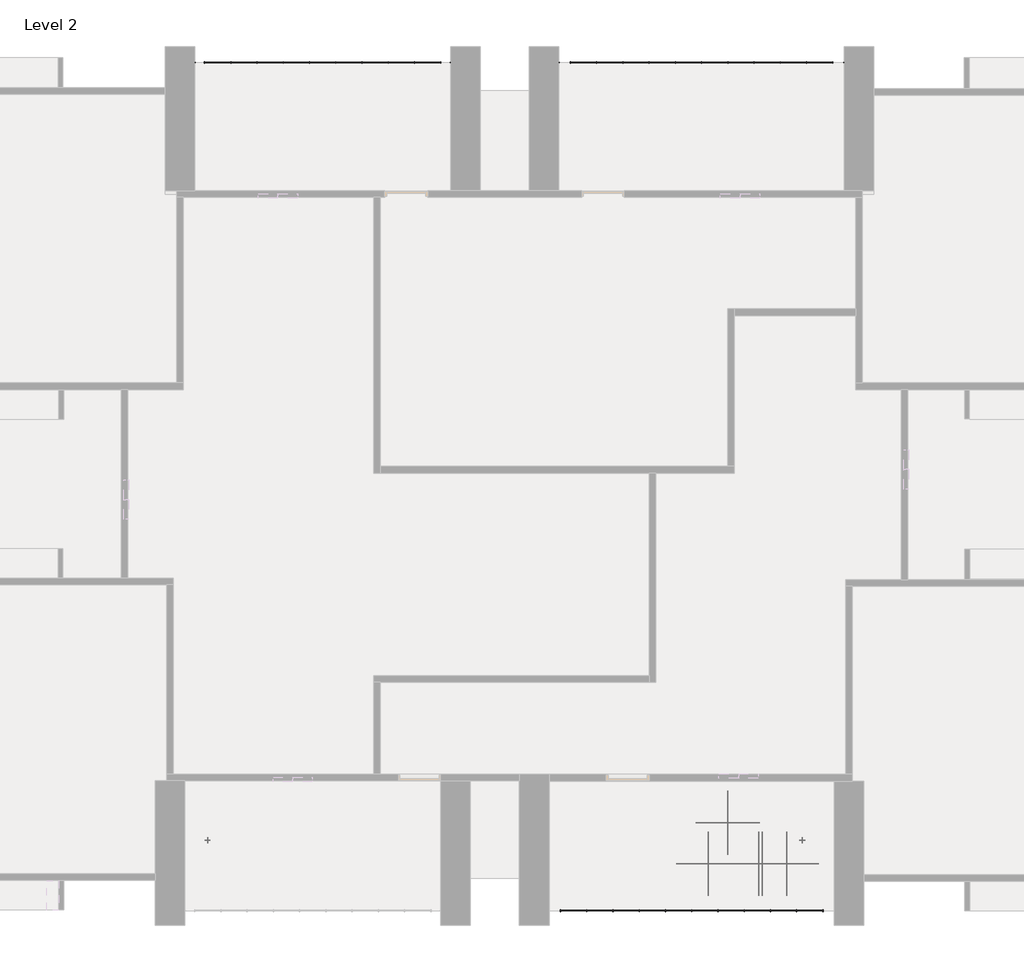
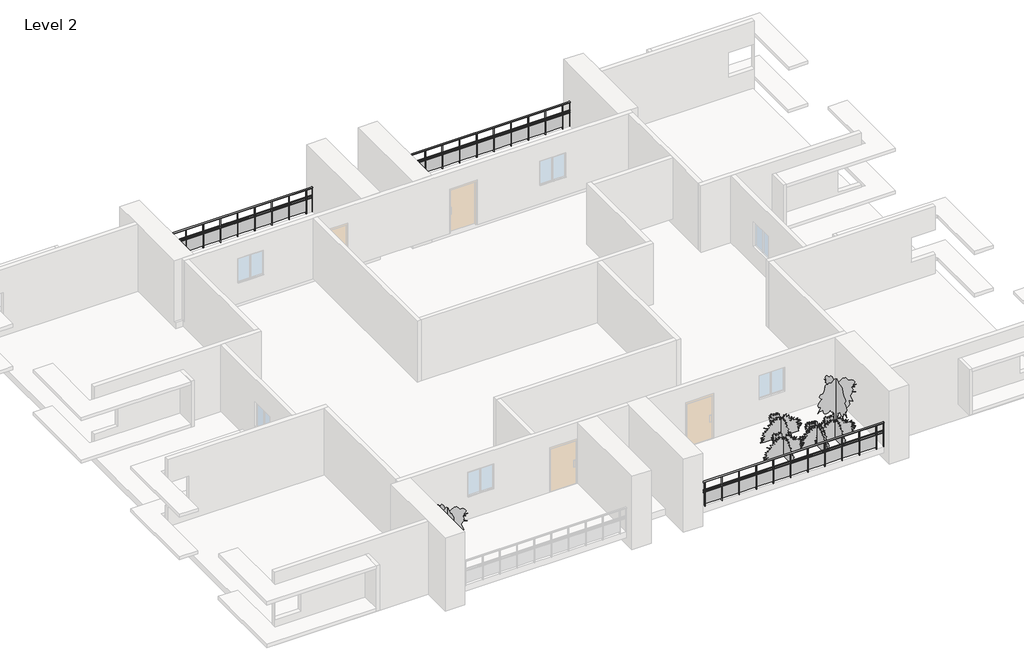
# One storey, part 4 of 4: 7 geographic elements, 3 railings.
"""IFC4 building model written with IfcOpenShell, lengths in millimetres."""

from ifc_helpers import new_model, si_unit, point, frame, origin, place, context, project, spatial, polyline, ellipse_curve, trimmed, outline, extrude, transform, mapped, element, save
from ifc_brep_helpers import plane_surface, extruded_surface, advanced_brep
from components import geographic_element_3d6ded1d, rpc_tree_tropical_d7a905c7

model = new_model("IFC4")

# Units and contexts
model_context = context("Model", 3, world=origin())
ifc_project = project(units=[si_unit("LENGTHUNIT", "METRE", prefix="MILLI")], contexts=[model_context])

# Site, building, storey
site = spatial("IfcSite", under=ifc_project)
building = spatial("IfcBuilding", under=site)
storey = spatial("IfcBuildingStorey", under=building, Name="Level 2", Elevation=3048.0)

# Geographic elements
placement = place(None, origin())
geographic_element_shape = geographic_element_3d6ded1d(model_context)
element("IfcGeographicElement", 1, ObjectType="RPC Shrub : Fountain Grass 3'-6\"", at=placement, inside=storey, context=model_context, shape_type="MappedRepresentation", body=[
    mapped(geographic_element_shape, transform((9500.2520665, -7929.230811, 3657.6), x_axis=(1.0, 0.0, 0.0), y_axis=(0.0, 1.0, 0.0), z_axis=(0.0, 0.0, 1.0))),
])
element("IfcGeographicElement", 2, ObjectType="RPC Shrub : Fountain Grass 3'-6\"", at=placement, inside=storey, context=model_context, shape_type="MappedRepresentation", body=[
    mapped(geographic_element_shape, transform((11938.6520665, -7929.230811, 3657.6), x_axis=(1.0, 0.0, 0.0), y_axis=(0.0, 1.0, 0.0), z_axis=(0.0, 0.0, 1.0))),
])
element("IfcGeographicElement", 3, ObjectType="RPC Shrub : Fountain Grass 3'-6\"", at=placement, inside=storey, context=model_context, shape_type="MappedRepresentation", body=[
    mapped(geographic_element_shape, transform((11176.6520665, -7929.230811, 3657.6), x_axis=(1.0, 0.0, 0.0), y_axis=(0.0, 1.0, 0.0), z_axis=(0.0, 0.0, 1.0))),
])
element("IfcGeographicElement", 4, ObjectType="RPC Shrub : Fountain Grass 3'-6\"", at=placement, inside=storey, context=model_context, shape_type="MappedRepresentation", body=[
    mapped(geographic_element_shape, transform((11075.0520665, -7929.230811, 3657.6), x_axis=(1.0, 0.0, 0.0), y_axis=(0.0, 1.0, 0.0), z_axis=(0.0, 0.0, 1.0))),
])
element("IfcGeographicElement", 5, ObjectType="RPC Shrub : Fountain Grass 3'-6\"", at=placement, inside=storey, context=model_context, shape_type="MappedRepresentation", body=[
    mapped(geographic_element_shape, transform((10109.8520665, -6659.230811, 3657.6), x_axis=(1.0, 0.0, 0.0), y_axis=(0.0, 1.0, 0.0), z_axis=(0.0, 0.0, 1.0))),
])
rpc_tree_tropical_shape = rpc_tree_tropical_d7a905c7(model_context)
element("IfcGeographicElement", 6, ObjectType="RPC Tree - Tropical", at=placement, inside=storey, context=model_context, shape_type="MappedRepresentation", body=[
    mapped(rpc_tree_tropical_shape, transform((-5993.7479335, -7192.630811, 3657.6), x_axis=(1.0, 0.0, 0.0), y_axis=(0.0, 1.0, 0.0), z_axis=(0.0, 0.0, 1.0))),
])
element("IfcGeographicElement", 7, ObjectType="RPC Tree - Tropical", at=placement, inside=storey, context=model_context, shape_type="MappedRepresentation", body=[
    mapped(rpc_tree_tropical_shape, transform((12421.2520665, -7192.630811, 3657.6), x_axis=(1.0, 0.0, 0.0), y_axis=(0.0, 1.0, 0.0), z_axis=(0.0, 0.0, 1.0))),
])

# Railings
element("IfcRailing", 8, ObjectType="Glass Panel - Bottom Fill", at=placement, inside=storey, context=model_context, shape_type="SolidModel", body=[
    advanced_brep(
    [(4572.6520665, -9342.282663, 4876.8), (4572.6520665, -9418.482663, 4876.8), (13411.8520665, -9342.282663, 4876.8), (13411.8520665, -9418.482663, 4876.8)],
    [
        (0, 1, ellipse_curve(frame((4572.6520665, -9380.382663, 4876.8), z_axis=(-1.0, 0.0, 0.0), x_axis=(0.0, -1.0, 0.0)), 38.1, 28.575)),
        (1, 0, ellipse_curve(frame((4572.6520665, -9380.382663, 4876.8), z_axis=(-1.0, 0.0, 0.0), x_axis=(0.0, -1.0, 0.0)), 38.1, 28.575)),
        (2, 3, ellipse_curve(frame((13411.8520665, -9380.382663, 4876.8), z_axis=(1.0, 0.0, 0.0), x_axis=(0.0, -1.0, 0.0)), 38.1, 28.575)),
        (3, 2, ellipse_curve(frame((13411.8520665, -9380.382663, 4876.8), z_axis=(1.0, 0.0, 0.0), x_axis=(0.0, -1.0, 0.0)), 38.1, 28.575)),
        (0, 2),
        (3, 1),
    ],
    [
        plane_surface(frame((4572.6520665, -9380.382663, 4876.8), z_axis=(-1.0, 0.0, 0.0), x_axis=(0.0, 1.0, 0.0))),
        plane_surface(frame((13411.8520665, -9380.382663, 4876.8), z_axis=(1.0, 0.0, 0.0), x_axis=(0.0, 1.0, 0.0))),
        extruded_surface(trimmed(ellipse_curve(frame((13411.8520665, -9380.382663, 4876.8), z_axis=(-1.0, 0.0, 0.0), x_axis=(0.0, -1.0, 0.0)), 38.1, 28.575), [point((13411.8520665, -9342.282663, 4876.8))], [point((13411.8520665, -9418.482663, 4876.8))], True, "CARTESIAN"), (-8839.2, 0.0, 0.0), 8839.2),
        extruded_surface(trimmed(ellipse_curve(frame((13411.8520665, -9380.382663, 4876.8), z_axis=(-1.0, 0.0, 0.0), x_axis=(0.0, -1.0, 0.0)), 38.1, 28.575), [point((13411.8520665, -9418.482663, 4876.8))], [point((13411.8520665, -9342.282663, 4876.8))], True, "CARTESIAN"), (-8839.2, 0.0, 0.0), 8839.2),
    ],
    [
        (0, [[1, 2]]),
        (1, [[3, 4]]),
        (2, [[-1, 5, -4, 6]]),
        (3, [[-2, -6, -3, -5]]),
    ],
),
    extrude(outline(polyline([(4572.6520665, -9393.082663), (4572.6520665, -9367.682663), (13411.8520665, -9367.682663), (13411.8520665, -9393.082663), (4572.6520665, -9393.082663)])), frame((0.0, 0.0, 4457.7), z_axis=(0.0, 0.0, 1.0), x_axis=(1.0, 0.0, 0.0)), (0.0, 0.0, 1.0), 25.4),
    extrude(outline(polyline([(4572.6520665, -9393.082663), (4572.6520665, -9367.682663), (13411.8520665, -9367.682663), (13411.8520665, -9393.082663), (4572.6520665, -9393.082663)])), frame((0.0, 0.0, 4356.1), z_axis=(0.0, 0.0, 1.0), x_axis=(1.0, 0.0, 0.0)), (0.0, 0.0, 1.0), 25.4),
    extrude(outline(polyline([(13049.9020665, -9405.782663), (13049.9020665, -9354.982663), (13062.6020665, -9354.982663), (13062.6020665, -9405.782663), (13049.9020665, -9405.782663)])), frame((0.0, 0.0, 3657.6), z_axis=(0.0, 0.0, 1.0), x_axis=(1.0, 0.0, 0.0)), (0.0, 0.0, 1.0), 1190.4788223),
    extrude(outline(polyline([(12243.4520665, -9373.847506), (13056.2520665, -9373.847506), (13056.2520665, -9380.197506), (12243.4520665, -9380.197506), (12243.4520665, -9373.847506)])), frame((0.0, 0.0, 3759.2), z_axis=(0.0, 0.0, 1.0), x_axis=(1.0, 0.0, 0.0)), (0.0, 0.0, 1.0), 596.9),
    extrude(outline(polyline([(12237.1020665, -9405.782663), (12237.1020665, -9354.982663), (12249.8020665, -9354.982663), (12249.8020665, -9405.782663), (12237.1020665, -9405.782663)])), frame((0.0, 0.0, 3657.6), z_axis=(0.0, 0.0, 1.0), x_axis=(1.0, 0.0, 0.0)), (0.0, 0.0, 1.0), 1190.4788223),
    extrude(outline(polyline([(11430.6520665, -9373.847506), (12243.4520665, -9373.847506), (12243.4520665, -9380.197506), (11430.6520665, -9380.197506), (11430.6520665, -9373.847506)])), frame((0.0, 0.0, 3759.2), z_axis=(0.0, 0.0, 1.0), x_axis=(1.0, 0.0, 0.0)), (0.0, 0.0, 1.0), 596.9),
    extrude(outline(polyline([(11424.3020665, -9405.782663), (11424.3020665, -9354.982663), (11437.0020665, -9354.982663), (11437.0020665, -9405.782663), (11424.3020665, -9405.782663)])), frame((0.0, 0.0, 3657.6), z_axis=(0.0, 0.0, 1.0), x_axis=(1.0, 0.0, 0.0)), (0.0, 0.0, 1.0), 1190.4788223),
    extrude(outline(polyline([(10617.8520665, -9373.847506), (11430.6520665, -9373.847506), (11430.6520665, -9380.197506), (10617.8520665, -9380.197506), (10617.8520665, -9373.847506)])), frame((0.0, 0.0, 3759.2), z_axis=(0.0, 0.0, 1.0), x_axis=(1.0, 0.0, 0.0)), (0.0, 0.0, 1.0), 596.9),
    extrude(outline(polyline([(10611.5020665, -9405.782663), (10611.5020665, -9354.982663), (10624.2020665, -9354.982663), (10624.2020665, -9405.782663), (10611.5020665, -9405.782663)])), frame((0.0, 0.0, 3657.6), z_axis=(0.0, 0.0, 1.0), x_axis=(1.0, 0.0, 0.0)), (0.0, 0.0, 1.0), 1190.4788223),
    extrude(outline(polyline([(9805.0520665, -9373.847506), (10617.8520665, -9373.847506), (10617.8520665, -9380.197506), (9805.0520665, -9380.197506), (9805.0520665, -9373.847506)])), frame((0.0, 0.0, 3759.2), z_axis=(0.0, 0.0, 1.0), x_axis=(1.0, 0.0, 0.0)), (0.0, 0.0, 1.0), 596.9),
    extrude(outline(polyline([(9798.7020665, -9405.782663), (9798.7020665, -9354.982663), (9811.4020665, -9354.982663), (9811.4020665, -9405.782663), (9798.7020665, -9405.782663)])), frame((0.0, 0.0, 3657.6), z_axis=(0.0, 0.0, 1.0), x_axis=(1.0, 0.0, 0.0)), (0.0, 0.0, 1.0), 1190.4788223),
    extrude(outline(polyline([(8992.2520665, -9373.847506), (9805.0520665, -9373.847506), (9805.0520665, -9380.197506), (8992.2520665, -9380.197506), (8992.2520665, -9373.847506)])), frame((0.0, 0.0, 3759.2), z_axis=(0.0, 0.0, 1.0), x_axis=(1.0, 0.0, 0.0)), (0.0, 0.0, 1.0), 596.9),
    extrude(outline(polyline([(8985.9020665, -9405.782663), (8985.9020665, -9354.982663), (8998.6020665, -9354.982663), (8998.6020665, -9405.782663), (8985.9020665, -9405.782663)])), frame((0.0, 0.0, 3657.6), z_axis=(0.0, 0.0, 1.0), x_axis=(1.0, 0.0, 0.0)), (0.0, 0.0, 1.0), 1190.4788223),
    extrude(outline(polyline([(8179.4520665, -9373.847506), (8992.2520665, -9373.847506), (8992.2520665, -9380.197506), (8179.4520665, -9380.197506), (8179.4520665, -9373.847506)])), frame((0.0, 0.0, 3759.2), z_axis=(0.0, 0.0, 1.0), x_axis=(1.0, 0.0, 0.0)), (0.0, 0.0, 1.0), 596.9),
    extrude(outline(polyline([(8173.1020665, -9405.782663), (8173.1020665, -9354.982663), (8185.8020665, -9354.982663), (8185.8020665, -9405.782663), (8173.1020665, -9405.782663)])), frame((0.0, 0.0, 3657.6), z_axis=(0.0, 0.0, 1.0), x_axis=(1.0, 0.0, 0.0)), (0.0, 0.0, 1.0), 1190.4788223),
    extrude(outline(polyline([(7366.6520665, -9373.847506), (8179.4520665, -9373.847506), (8179.4520665, -9380.197506), (7366.6520665, -9380.197506), (7366.6520665, -9373.847506)])), frame((0.0, 0.0, 3759.2), z_axis=(0.0, 0.0, 1.0), x_axis=(1.0, 0.0, 0.0)), (0.0, 0.0, 1.0), 596.9),
    extrude(outline(polyline([(7360.3020665, -9405.782663), (7360.3020665, -9354.982663), (7373.0020665, -9354.982663), (7373.0020665, -9405.782663), (7360.3020665, -9405.782663)])), frame((0.0, 0.0, 3657.6), z_axis=(0.0, 0.0, 1.0), x_axis=(1.0, 0.0, 0.0)), (0.0, 0.0, 1.0), 1190.4788223),
    extrude(outline(polyline([(6553.8520665, -9373.847506), (7366.6520665, -9373.847506), (7366.6520665, -9380.197506), (6553.8520665, -9380.197506), (6553.8520665, -9373.847506)])), frame((0.0, 0.0, 3759.2), z_axis=(0.0, 0.0, 1.0), x_axis=(1.0, 0.0, 0.0)), (0.0, 0.0, 1.0), 596.9),
    extrude(outline(polyline([(6547.5020665, -9405.782663), (6547.5020665, -9354.982663), (6560.2020665, -9354.982663), (6560.2020665, -9405.782663), (6547.5020665, -9405.782663)])), frame((0.0, 0.0, 3657.6), z_axis=(0.0, 0.0, 1.0), x_axis=(1.0, 0.0, 0.0)), (0.0, 0.0, 1.0), 1190.4788223),
    extrude(outline(polyline([(5741.0520665, -9373.847506), (6553.8520665, -9373.847506), (6553.8520665, -9380.197506), (5741.0520665, -9380.197506), (5741.0520665, -9373.847506)])), frame((0.0, 0.0, 3759.2), z_axis=(0.0, 0.0, 1.0), x_axis=(1.0, 0.0, 0.0)), (0.0, 0.0, 1.0), 596.9),
    extrude(outline(polyline([(5734.7020665, -9405.782663), (5734.7020665, -9354.982663), (5747.4020665, -9354.982663), (5747.4020665, -9405.782663), (5734.7020665, -9405.782663)])), frame((0.0, 0.0, 3657.6), z_axis=(0.0, 0.0, 1.0), x_axis=(1.0, 0.0, 0.0)), (0.0, 0.0, 1.0), 1190.4788223),
    extrude(outline(polyline([(4928.2520665, -9373.847506), (5741.0520665, -9373.847506), (5741.0520665, -9380.197506), (4928.2520665, -9380.197506), (4928.2520665, -9373.847506)])), frame((0.0, 0.0, 3759.2), z_axis=(0.0, 0.0, 1.0), x_axis=(1.0, 0.0, 0.0)), (0.0, 0.0, 1.0), 596.9),
    extrude(outline(polyline([(4921.9020665, -9405.782663), (4921.9020665, -9354.982663), (4934.6020665, -9354.982663), (4934.6020665, -9405.782663), (4921.9020665, -9405.782663)])), frame((0.0, 0.0, 3657.6), z_axis=(0.0, 0.0, 1.0), x_axis=(1.0, 0.0, 0.0)), (0.0, 0.0, 1.0), 1190.4788223),
    extrude(outline(polyline([(13399.1520665, -9389.907663), (13399.1520665, -9370.857663), (13418.2020665, -9370.857663), (13418.2020665, -9389.907663), (13399.1520665, -9389.907663)])), frame((0.0, 0.0, 3657.6), z_axis=(0.0, 0.0, 1.0), x_axis=(1.0, 0.0, 0.0)), (0.0, 0.0, 1.0), 1190.4788223),
    extrude(outline(polyline([(4566.3020665, -9389.907663), (4566.3020665, -9370.857663), (4585.3520665, -9370.857663), (4585.3520665, -9389.907663), (4566.3020665, -9389.907663)])), frame((0.0, 0.0, 3657.6), z_axis=(0.0, 0.0, 1.0), x_axis=(1.0, 0.0, 0.0)), (0.0, 0.0, 1.0), 1190.4788223),
])
element("IfcRailing", 9, ObjectType="Glass Panel - Bottom Fill", at=placement, inside=storey, context=model_context, shape_type="SolidModel", body=[
    advanced_brep(
    [(-6400.1479335, 16924.2559451, 4876.8), (-6400.1479335, 16848.0559451, 4876.8), (1524.6520665, 16924.2559451, 4876.8), (1524.6520665, 16848.0559451, 4876.8)],
    [
        (0, 1, ellipse_curve(frame((-6400.1479335, 16886.1559451, 4876.8), z_axis=(-1.0, 0.0, 0.0), x_axis=(0.0, -1.0, 0.0)), 38.1, 28.575)),
        (1, 0, ellipse_curve(frame((-6400.1479335, 16886.1559451, 4876.8), z_axis=(-1.0, 0.0, 0.0), x_axis=(0.0, -1.0, 0.0)), 38.1, 28.575)),
        (2, 3, ellipse_curve(frame((1524.6520665, 16886.1559451, 4876.8), z_axis=(1.0, 0.0, 0.0), x_axis=(0.0, -1.0, 0.0)), 38.1, 28.575)),
        (3, 2, ellipse_curve(frame((1524.6520665, 16886.1559451, 4876.8), z_axis=(1.0, 0.0, 0.0), x_axis=(0.0, -1.0, 0.0)), 38.1, 28.575)),
        (0, 2),
        (3, 1),
    ],
    [
        plane_surface(frame((-6400.1479335, 16886.1559451, 4876.8), z_axis=(-1.0, 0.0, 0.0), x_axis=(0.0, 1.0, 0.0))),
        plane_surface(frame((1524.6520665, 16886.1559451, 4876.8), z_axis=(1.0, 0.0, 0.0), x_axis=(0.0, 1.0, 0.0))),
        extruded_surface(trimmed(ellipse_curve(frame((1524.6520665, 16886.1559451, 4876.8), z_axis=(-1.0, 0.0, 0.0), x_axis=(0.0, -1.0, 0.0)), 38.1, 28.575), [point((1524.6520665, 16924.2559451, 4876.8))], [point((1524.6520665, 16848.0559451, 4876.8))], True, "CARTESIAN"), (-7924.8, 0.0, 0.0), 7924.8),
        extruded_surface(trimmed(ellipse_curve(frame((1524.6520665, 16886.1559451, 4876.8), z_axis=(-1.0, 0.0, 0.0), x_axis=(0.0, -1.0, 0.0)), 38.1, 28.575), [point((1524.6520665, 16848.0559451, 4876.8))], [point((1524.6520665, 16924.2559451, 4876.8))], True, "CARTESIAN"), (-7924.8, 0.0, 0.0), 7924.8),
    ],
    [
        (0, [[1, 2]]),
        (1, [[3, 4]]),
        (2, [[-1, 5, -4, 6]]),
        (3, [[-2, -6, -3, -5]]),
    ],
),
    extrude(outline(polyline([(-6400.1479335, 16873.4559451), (-6400.1479335, 16898.8559451), (1524.6520665, 16898.8559451), (1524.6520665, 16873.4559451), (-6400.1479335, 16873.4559451)])), frame((0.0, 0.0, 4457.7), z_axis=(0.0, 0.0, 1.0), x_axis=(1.0, 0.0, 0.0)), (0.0, 0.0, 1.0), 25.4),
    extrude(outline(polyline([(-6400.1479335, 16873.4559451), (-6400.1479335, 16898.8559451), (1524.6520665, 16898.8559451), (1524.6520665, 16873.4559451), (-6400.1479335, 16873.4559451)])), frame((0.0, 0.0, 4356.1), z_axis=(0.0, 0.0, 1.0), x_axis=(1.0, 0.0, 0.0)), (0.0, 0.0, 1.0), 25.4),
    extrude(outline(polyline([(1213.5020665, 16860.7559451), (1213.5020665, 16911.5559451), (1226.2020665, 16911.5559451), (1226.2020665, 16860.7559451), (1213.5020665, 16860.7559451)])), frame((0.0, 0.0, 3657.6), z_axis=(0.0, 0.0, 1.0), x_axis=(1.0, 0.0, 0.0)), (0.0, 0.0, 1.0), 1190.4788223),
    extrude(outline(polyline([(407.0520665, 16892.6911021), (1219.8520665, 16892.6911021), (1219.8520665, 16886.3411021), (407.0520665, 16886.3411021), (407.0520665, 16892.6911021)])), frame((0.0, 0.0, 3759.2), z_axis=(0.0, 0.0, 1.0), x_axis=(1.0, 0.0, 0.0)), (0.0, 0.0, 1.0), 596.9),
    extrude(outline(polyline([(400.7020665, 16860.7559451), (400.7020665, 16911.5559451), (413.4020665, 16911.5559451), (413.4020665, 16860.7559451), (400.7020665, 16860.7559451)])), frame((0.0, 0.0, 3657.6), z_axis=(0.0, 0.0, 1.0), x_axis=(1.0, 0.0, 0.0)), (0.0, 0.0, 1.0), 1190.4788223),
    extrude(outline(polyline([(-405.7479335, 16892.6911021), (407.0520665, 16892.6911021), (407.0520665, 16886.3411021), (-405.7479335, 16886.3411021), (-405.7479335, 16892.6911021)])), frame((0.0, 0.0, 3759.2), z_axis=(0.0, 0.0, 1.0), x_axis=(1.0, 0.0, 0.0)), (0.0, 0.0, 1.0), 596.9),
    extrude(outline(polyline([(-412.0979335, 16860.7559451), (-412.0979335, 16911.5559451), (-399.3979335, 16911.5559451), (-399.3979335, 16860.7559451), (-412.0979335, 16860.7559451)])), frame((0.0, 0.0, 3657.6), z_axis=(0.0, 0.0, 1.0), x_axis=(1.0, 0.0, 0.0)), (0.0, 0.0, 1.0), 1190.4788223),
    extrude(outline(polyline([(-1218.5479335, 16892.6911021), (-405.7479335, 16892.6911021), (-405.7479335, 16886.3411021), (-1218.5479335, 16886.3411021), (-1218.5479335, 16892.6911021)])), frame((0.0, 0.0, 3759.2), z_axis=(0.0, 0.0, 1.0), x_axis=(1.0, 0.0, 0.0)), (0.0, 0.0, 1.0), 596.9),
    extrude(outline(polyline([(-1224.8979335, 16860.7559451), (-1224.8979335, 16911.5559451), (-1212.1979335, 16911.5559451), (-1212.1979335, 16860.7559451), (-1224.8979335, 16860.7559451)])), frame((0.0, 0.0, 3657.6), z_axis=(0.0, 0.0, 1.0), x_axis=(1.0, 0.0, 0.0)), (0.0, 0.0, 1.0), 1190.4788223),
    extrude(outline(polyline([(-2031.3479335, 16892.6911021), (-1218.5479335, 16892.6911021), (-1218.5479335, 16886.3411021), (-2031.3479335, 16886.3411021), (-2031.3479335, 16892.6911021)])), frame((0.0, 0.0, 3759.2), z_axis=(0.0, 0.0, 1.0), x_axis=(1.0, 0.0, 0.0)), (0.0, 0.0, 1.0), 596.9),
    extrude(outline(polyline([(-2037.6979335, 16860.7559451), (-2037.6979335, 16911.5559451), (-2024.9979335, 16911.5559451), (-2024.9979335, 16860.7559451), (-2037.6979335, 16860.7559451)])), frame((0.0, 0.0, 3657.6), z_axis=(0.0, 0.0, 1.0), x_axis=(1.0, 0.0, 0.0)), (0.0, 0.0, 1.0), 1190.4788223),
    extrude(outline(polyline([(-2844.1479335, 16892.6911021), (-2031.3479335, 16892.6911021), (-2031.3479335, 16886.3411021), (-2844.1479335, 16886.3411021), (-2844.1479335, 16892.6911021)])), frame((0.0, 0.0, 3759.2), z_axis=(0.0, 0.0, 1.0), x_axis=(1.0, 0.0, 0.0)), (0.0, 0.0, 1.0), 596.9),
    extrude(outline(polyline([(-2850.4979335, 16860.7559451), (-2850.4979335, 16911.5559451), (-2837.7979335, 16911.5559451), (-2837.7979335, 16860.7559451), (-2850.4979335, 16860.7559451)])), frame((0.0, 0.0, 3657.6), z_axis=(0.0, 0.0, 1.0), x_axis=(1.0, 0.0, 0.0)), (0.0, 0.0, 1.0), 1190.4788223),
    extrude(outline(polyline([(-3656.9479335, 16892.6911021), (-2844.1479335, 16892.6911021), (-2844.1479335, 16886.3411021), (-3656.9479335, 16886.3411021), (-3656.9479335, 16892.6911021)])), frame((0.0, 0.0, 3759.2), z_axis=(0.0, 0.0, 1.0), x_axis=(1.0, 0.0, 0.0)), (0.0, 0.0, 1.0), 596.9),
    extrude(outline(polyline([(-3663.2979335, 16860.7559451), (-3663.2979335, 16911.5559451), (-3650.5979335, 16911.5559451), (-3650.5979335, 16860.7559451), (-3663.2979335, 16860.7559451)])), frame((0.0, 0.0, 3657.6), z_axis=(0.0, 0.0, 1.0), x_axis=(1.0, 0.0, 0.0)), (0.0, 0.0, 1.0), 1190.4788223),
    extrude(outline(polyline([(-4469.7479335, 16892.6911021), (-3656.9479335, 16892.6911021), (-3656.9479335, 16886.3411021), (-4469.7479335, 16886.3411021), (-4469.7479335, 16892.6911021)])), frame((0.0, 0.0, 3759.2), z_axis=(0.0, 0.0, 1.0), x_axis=(1.0, 0.0, 0.0)), (0.0, 0.0, 1.0), 596.9),
    extrude(outline(polyline([(-4476.0979335, 16860.7559451), (-4476.0979335, 16911.5559451), (-4463.3979335, 16911.5559451), (-4463.3979335, 16860.7559451), (-4476.0979335, 16860.7559451)])), frame((0.0, 0.0, 3657.6), z_axis=(0.0, 0.0, 1.0), x_axis=(1.0, 0.0, 0.0)), (0.0, 0.0, 1.0), 1190.4788223),
    extrude(outline(polyline([(-5282.5479335, 16892.6911021), (-4469.7479335, 16892.6911021), (-4469.7479335, 16886.3411021), (-5282.5479335, 16886.3411021), (-5282.5479335, 16892.6911021)])), frame((0.0, 0.0, 3759.2), z_axis=(0.0, 0.0, 1.0), x_axis=(1.0, 0.0, 0.0)), (0.0, 0.0, 1.0), 596.9),
    extrude(outline(polyline([(-5288.8979335, 16860.7559451), (-5288.8979335, 16911.5559451), (-5276.1979335, 16911.5559451), (-5276.1979335, 16860.7559451), (-5288.8979335, 16860.7559451)])), frame((0.0, 0.0, 3657.6), z_axis=(0.0, 0.0, 1.0), x_axis=(1.0, 0.0, 0.0)), (0.0, 0.0, 1.0), 1190.4788223),
    extrude(outline(polyline([(-6095.3479335, 16892.6911021), (-5282.5479335, 16892.6911021), (-5282.5479335, 16886.3411021), (-6095.3479335, 16886.3411021), (-6095.3479335, 16892.6911021)])), frame((0.0, 0.0, 3759.2), z_axis=(0.0, 0.0, 1.0), x_axis=(1.0, 0.0, 0.0)), (0.0, 0.0, 1.0), 596.9),
    extrude(outline(polyline([(-6101.6979335, 16860.7559451), (-6101.6979335, 16911.5559451), (-6088.9979335, 16911.5559451), (-6088.9979335, 16860.7559451), (-6101.6979335, 16860.7559451)])), frame((0.0, 0.0, 3657.6), z_axis=(0.0, 0.0, 1.0), x_axis=(1.0, 0.0, 0.0)), (0.0, 0.0, 1.0), 1190.4788223),
    extrude(outline(polyline([(1511.9520665, 16876.6309451), (1511.9520665, 16895.6809451), (1531.0020665, 16895.6809451), (1531.0020665, 16876.6309451), (1511.9520665, 16876.6309451)])), frame((0.0, 0.0, 3657.6), z_axis=(0.0, 0.0, 1.0), x_axis=(1.0, 0.0, 0.0)), (0.0, 0.0, 1.0), 1190.4788223),
    extrude(outline(polyline([(-6406.4979335, 16876.6309451), (-6406.4979335, 16895.6809451), (-6387.4479335, 16895.6809451), (-6387.4479335, 16876.6309451), (-6406.4979335, 16876.6309451)])), frame((0.0, 0.0, 3657.6), z_axis=(0.0, 0.0, 1.0), x_axis=(1.0, 0.0, 0.0)), (0.0, 0.0, 1.0), 1190.4788223),
])
element("IfcRailing", 10, ObjectType="Glass Panel - Bottom Fill", at=placement, inside=storey, context=model_context, shape_type="SolidModel", body=[
    advanced_brep(
    [(4877.4520665, 16924.2559451, 4876.8), (4877.4520665, 16848.0559451, 4876.8), (13716.6520665, 16924.2559451, 4876.8), (13716.6520665, 16848.0559451, 4876.8)],
    [
        (0, 1, ellipse_curve(frame((4877.4520665, 16886.1559451, 4876.8), z_axis=(-1.0, 0.0, 0.0), x_axis=(0.0, -1.0, 0.0)), 38.1, 28.575)),
        (1, 0, ellipse_curve(frame((4877.4520665, 16886.1559451, 4876.8), z_axis=(-1.0, 0.0, 0.0), x_axis=(0.0, -1.0, 0.0)), 38.1, 28.575)),
        (2, 3, ellipse_curve(frame((13716.6520665, 16886.1559451, 4876.8), z_axis=(1.0, 0.0, 0.0), x_axis=(0.0, -1.0, 0.0)), 38.1, 28.575)),
        (3, 2, ellipse_curve(frame((13716.6520665, 16886.1559451, 4876.8), z_axis=(1.0, 0.0, 0.0), x_axis=(0.0, -1.0, 0.0)), 38.1, 28.575)),
        (0, 2),
        (3, 1),
    ],
    [
        plane_surface(frame((4877.4520665, 16886.1559451, 4876.8), z_axis=(-1.0, 0.0, 0.0), x_axis=(0.0, 1.0, 0.0))),
        plane_surface(frame((13716.6520665, 16886.1559451, 4876.8), z_axis=(1.0, 0.0, 0.0), x_axis=(0.0, 1.0, 0.0))),
        extruded_surface(trimmed(ellipse_curve(frame((13716.6520665, 16886.1559451, 4876.8), z_axis=(-1.0, 0.0, 0.0), x_axis=(0.0, -1.0, 0.0)), 38.1, 28.575), [point((13716.6520665, 16924.2559451, 4876.8))], [point((13716.6520665, 16848.0559451, 4876.8))], True, "CARTESIAN"), (-8839.2, 0.0, 0.0), 8839.2),
        extruded_surface(trimmed(ellipse_curve(frame((13716.6520665, 16886.1559451, 4876.8), z_axis=(-1.0, 0.0, 0.0), x_axis=(0.0, -1.0, 0.0)), 38.1, 28.575), [point((13716.6520665, 16848.0559451, 4876.8))], [point((13716.6520665, 16924.2559451, 4876.8))], True, "CARTESIAN"), (-8839.2, 0.0, 0.0), 8839.2),
    ],
    [
        (0, [[1, 2]]),
        (1, [[3, 4]]),
        (2, [[-1, 5, -4, 6]]),
        (3, [[-2, -6, -3, -5]]),
    ],
),
    extrude(outline(polyline([(4877.4520665, 16873.4559451), (4877.4520665, 16898.8559451), (13716.6520665, 16898.8559451), (13716.6520665, 16873.4559451), (4877.4520665, 16873.4559451)])), frame((0.0, 0.0, 4457.7), z_axis=(0.0, 0.0, 1.0), x_axis=(1.0, 0.0, 0.0)), (0.0, 0.0, 1.0), 25.4),
    extrude(outline(polyline([(4877.4520665, 16873.4559451), (4877.4520665, 16898.8559451), (13716.6520665, 16898.8559451), (13716.6520665, 16873.4559451), (4877.4520665, 16873.4559451)])), frame((0.0, 0.0, 4356.1), z_axis=(0.0, 0.0, 1.0), x_axis=(1.0, 0.0, 0.0)), (0.0, 0.0, 1.0), 25.4),
    extrude(outline(polyline([(13354.7020665, 16860.7559451), (13354.7020665, 16911.5559451), (13367.4020665, 16911.5559451), (13367.4020665, 16860.7559451), (13354.7020665, 16860.7559451)])), frame((0.0, 0.0, 3657.6), z_axis=(0.0, 0.0, 1.0), x_axis=(1.0, 0.0, 0.0)), (0.0, 0.0, 1.0), 1190.4788223),
    extrude(outline(polyline([(12548.2520665, 16892.6911021), (13361.0520665, 16892.6911021), (13361.0520665, 16886.3411021), (12548.2520665, 16886.3411021), (12548.2520665, 16892.6911021)])), frame((0.0, 0.0, 3759.2), z_axis=(0.0, 0.0, 1.0), x_axis=(1.0, 0.0, 0.0)), (0.0, 0.0, 1.0), 596.9),
    extrude(outline(polyline([(12541.9020665, 16860.7559451), (12541.9020665, 16911.5559451), (12554.6020665, 16911.5559451), (12554.6020665, 16860.7559451), (12541.9020665, 16860.7559451)])), frame((0.0, 0.0, 3657.6), z_axis=(0.0, 0.0, 1.0), x_axis=(1.0, 0.0, 0.0)), (0.0, 0.0, 1.0), 1190.4788223),
    extrude(outline(polyline([(11735.4520665, 16892.6911021), (12548.2520665, 16892.6911021), (12548.2520665, 16886.3411021), (11735.4520665, 16886.3411021), (11735.4520665, 16892.6911021)])), frame((0.0, 0.0, 3759.2), z_axis=(0.0, 0.0, 1.0), x_axis=(1.0, 0.0, 0.0)), (0.0, 0.0, 1.0), 596.9),
    extrude(outline(polyline([(11729.1020665, 16860.7559451), (11729.1020665, 16911.5559451), (11741.8020665, 16911.5559451), (11741.8020665, 16860.7559451), (11729.1020665, 16860.7559451)])), frame((0.0, 0.0, 3657.6), z_axis=(0.0, 0.0, 1.0), x_axis=(1.0, 0.0, 0.0)), (0.0, 0.0, 1.0), 1190.4788223),
    extrude(outline(polyline([(10922.6520665, 16892.6911021), (11735.4520665, 16892.6911021), (11735.4520665, 16886.3411021), (10922.6520665, 16886.3411021), (10922.6520665, 16892.6911021)])), frame((0.0, 0.0, 3759.2), z_axis=(0.0, 0.0, 1.0), x_axis=(1.0, 0.0, 0.0)), (0.0, 0.0, 1.0), 596.9),
    extrude(outline(polyline([(10916.3020665, 16860.7559451), (10916.3020665, 16911.5559451), (10929.0020665, 16911.5559451), (10929.0020665, 16860.7559451), (10916.3020665, 16860.7559451)])), frame((0.0, 0.0, 3657.6), z_axis=(0.0, 0.0, 1.0), x_axis=(1.0, 0.0, 0.0)), (0.0, 0.0, 1.0), 1190.4788223),
    extrude(outline(polyline([(10109.8520665, 16892.6911021), (10922.6520665, 16892.6911021), (10922.6520665, 16886.3411021), (10109.8520665, 16886.3411021), (10109.8520665, 16892.6911021)])), frame((0.0, 0.0, 3759.2), z_axis=(0.0, 0.0, 1.0), x_axis=(1.0, 0.0, 0.0)), (0.0, 0.0, 1.0), 596.9),
    extrude(outline(polyline([(10103.5020665, 16860.7559451), (10103.5020665, 16911.5559451), (10116.2020665, 16911.5559451), (10116.2020665, 16860.7559451), (10103.5020665, 16860.7559451)])), frame((0.0, 0.0, 3657.6), z_axis=(0.0, 0.0, 1.0), x_axis=(1.0, 0.0, 0.0)), (0.0, 0.0, 1.0), 1190.4788223),
    extrude(outline(polyline([(9297.0520665, 16892.6911021), (10109.8520665, 16892.6911021), (10109.8520665, 16886.3411021), (9297.0520665, 16886.3411021), (9297.0520665, 16892.6911021)])), frame((0.0, 0.0, 3759.2), z_axis=(0.0, 0.0, 1.0), x_axis=(1.0, 0.0, 0.0)), (0.0, 0.0, 1.0), 596.9),
    extrude(outline(polyline([(9290.7020665, 16860.7559451), (9290.7020665, 16911.5559451), (9303.4020665, 16911.5559451), (9303.4020665, 16860.7559451), (9290.7020665, 16860.7559451)])), frame((0.0, 0.0, 3657.6), z_axis=(0.0, 0.0, 1.0), x_axis=(1.0, 0.0, 0.0)), (0.0, 0.0, 1.0), 1190.4788223),
    extrude(outline(polyline([(8484.2520665, 16892.6911021), (9297.0520665, 16892.6911021), (9297.0520665, 16886.3411021), (8484.2520665, 16886.3411021), (8484.2520665, 16892.6911021)])), frame((0.0, 0.0, 3759.2), z_axis=(0.0, 0.0, 1.0), x_axis=(1.0, 0.0, 0.0)), (0.0, 0.0, 1.0), 596.9),
    extrude(outline(polyline([(8477.9020665, 16860.7559451), (8477.9020665, 16911.5559451), (8490.6020665, 16911.5559451), (8490.6020665, 16860.7559451), (8477.9020665, 16860.7559451)])), frame((0.0, 0.0, 3657.6), z_axis=(0.0, 0.0, 1.0), x_axis=(1.0, 0.0, 0.0)), (0.0, 0.0, 1.0), 1190.4788223),
    extrude(outline(polyline([(7671.4520665, 16892.6911021), (8484.2520665, 16892.6911021), (8484.2520665, 16886.3411021), (7671.4520665, 16886.3411021), (7671.4520665, 16892.6911021)])), frame((0.0, 0.0, 3759.2), z_axis=(0.0, 0.0, 1.0), x_axis=(1.0, 0.0, 0.0)), (0.0, 0.0, 1.0), 596.9),
    extrude(outline(polyline([(7665.1020665, 16860.7559451), (7665.1020665, 16911.5559451), (7677.8020665, 16911.5559451), (7677.8020665, 16860.7559451), (7665.1020665, 16860.7559451)])), frame((0.0, 0.0, 3657.6), z_axis=(0.0, 0.0, 1.0), x_axis=(1.0, 0.0, 0.0)), (0.0, 0.0, 1.0), 1190.4788223),
    extrude(outline(polyline([(6858.6520665, 16892.6911021), (7671.4520665, 16892.6911021), (7671.4520665, 16886.3411021), (6858.6520665, 16886.3411021), (6858.6520665, 16892.6911021)])), frame((0.0, 0.0, 3759.2), z_axis=(0.0, 0.0, 1.0), x_axis=(1.0, 0.0, 0.0)), (0.0, 0.0, 1.0), 596.9),
    extrude(outline(polyline([(6852.3020665, 16860.7559451), (6852.3020665, 16911.5559451), (6865.0020665, 16911.5559451), (6865.0020665, 16860.7559451), (6852.3020665, 16860.7559451)])), frame((0.0, 0.0, 3657.6), z_axis=(0.0, 0.0, 1.0), x_axis=(1.0, 0.0, 0.0)), (0.0, 0.0, 1.0), 1190.4788223),
    extrude(outline(polyline([(6045.8520665, 16892.6911021), (6858.6520665, 16892.6911021), (6858.6520665, 16886.3411021), (6045.8520665, 16886.3411021), (6045.8520665, 16892.6911021)])), frame((0.0, 0.0, 3759.2), z_axis=(0.0, 0.0, 1.0), x_axis=(1.0, 0.0, 0.0)), (0.0, 0.0, 1.0), 596.9),
    extrude(outline(polyline([(6039.5020665, 16860.7559451), (6039.5020665, 16911.5559451), (6052.2020665, 16911.5559451), (6052.2020665, 16860.7559451), (6039.5020665, 16860.7559451)])), frame((0.0, 0.0, 3657.6), z_axis=(0.0, 0.0, 1.0), x_axis=(1.0, 0.0, 0.0)), (0.0, 0.0, 1.0), 1190.4788223),
    extrude(outline(polyline([(5233.0520665, 16892.6911021), (6045.8520665, 16892.6911021), (6045.8520665, 16886.3411021), (5233.0520665, 16886.3411021), (5233.0520665, 16892.6911021)])), frame((0.0, 0.0, 3759.2), z_axis=(0.0, 0.0, 1.0), x_axis=(1.0, 0.0, 0.0)), (0.0, 0.0, 1.0), 596.9),
    extrude(outline(polyline([(5226.7020665, 16860.7559451), (5226.7020665, 16911.5559451), (5239.4020665, 16911.5559451), (5239.4020665, 16860.7559451), (5226.7020665, 16860.7559451)])), frame((0.0, 0.0, 3657.6), z_axis=(0.0, 0.0, 1.0), x_axis=(1.0, 0.0, 0.0)), (0.0, 0.0, 1.0), 1190.4788223),
    extrude(outline(polyline([(13703.9520665, 16876.6309451), (13703.9520665, 16895.6809451), (13723.0020665, 16895.6809451), (13723.0020665, 16876.6309451), (13703.9520665, 16876.6309451)])), frame((0.0, 0.0, 3657.6), z_axis=(0.0, 0.0, 1.0), x_axis=(1.0, 0.0, 0.0)), (0.0, 0.0, 1.0), 1190.4788223),
    extrude(outline(polyline([(4871.1020665, 16876.6309451), (4871.1020665, 16895.6809451), (4890.1520665, 16895.6809451), (4890.1520665, 16876.6309451), (4871.1020665, 16876.6309451)])), frame((0.0, 0.0, 3657.6), z_axis=(0.0, 0.0, 1.0), x_axis=(1.0, 0.0, 0.0)), (0.0, 0.0, 1.0), 1190.4788223),
])

save(model, "model.ifc")

# Revit data of these elements
# Type "RPC Shrub : Fountain Grass 3'-6\""
#   Type Comments = "Fountain Grass"
#   built-in parameter 1005198 = "{2, 15},{39, RPC-16-G1GP-21FX-7KGL-L000-ST1L-LVER-AU},{1, 0},{1, 0},{2, 13},{1, 8},{5, Color},{1, 0},{1, 0},{3, 0.8},{3, 0.8},{3, 0.8},{1, 8},{7, BBoxMin},{1, 0},{1, 0},{1, 0},{1, 0},{1, 0},{1, 8},{7, BBoxMax},{1, 0},{1, 0},{1, 0},{1, 0},{1, 0},{2, 11},{9, RPCTypeId},{1, 0},{1, 0},{39, RPC-16-G1GP-21FX-7KGL-L000-ST1L-LVER-AU},{1, 6},{14, RPCPlantHeight},{1, 0},{1, 0},{3, 3.5},{2, 11},{7, keyword},{1, 0},{1, 0},{35, :RPCs:Shrubs & Grasses:Geometry:RPC},{2, 11},{8, category},{1, 0},{1, 0},{16, Shrubs & Grasses},{2, 11},{12, LocalizedUID},{1, 0},{1, 0},{14, Fountain Grass},{2, 14},{6, Height},{1, 0},{1, 0},{3, 3.5},{1, 2},{16, Cast Reflections},{1, 0},{1, 0},{1, 0},{1, 2},{12, Cast Shadows},{1, 0},{1, 0},{1, 1},{1, 2},{9, Lock View},{1, 0},{1, 0},{1, 0},{1, 4},{5, ViewC},{1, 0},{1, 0},{1, 0},{21, assetlibrary_base.fbx},{1, 5},"
#   built-in parameter 1005195 = "RPC-16-G1GP-21FX-7KGL-L000-ST1L-LVER-AU"
#   Assembly Code = "G2050500"
#   Height = 3' - 6"
#   Default Elevation = 0
# Type "RPC Tree - Tropical"
#   built-in parameter 1005198 = "{2, 15},{39, RPC-16-G2MF-J1Q0-CAN1-N000-ST1L-LVER-AU},{1, 0},{1, 0},{2, 13},{1, 8},{5, Color},{1, 0},{1, 0},{3, 0.8},{3, 0.8},{3, 0.8},{1, 8},{7, BBoxMin},{1, 0},{1, 0},{1, 0},{1, 0},{1, 0},{1, 8},{7, BBoxMax},{1, 0},{1, 0},{1, 0},{1, 0},{1, 0},{2, 11},{9, RPCTypeId},{1, 0},{1, 0},{39, RPC-16-G2MF-J1Q0-CAN1-N000-ST1L-LVER-AU},{1, 6},{14, RPCPlantHeight},{1, 0},{1, 0},{1, 8},{2, 11},{7, keyword},{1, 0},{1, 0},{35, :RPCs:Trees [Tropical]:Geometry:RPC},{2, 11},{8, category},{1, 0},{1, 0},{16, Trees [Tropical]},{2, 11},{12, LocalizedUID},{1, 0},{1, 0},{13, Windmill Palm},{2, 14},{6, Height},{1, 0},{1, 0},{1, 8},{1, 2},{16, Cast Reflections},{1, 0},{1, 0},{1, 0},{1, 2},{12, Cast Shadows},{1, 0},{1, 0},{1, 1},{1, 2},{9, Lock View},{1, 0},{1, 0},{1, 0},{1, 4},{5, ViewC},{1, 0},{1, 0},{1, 0},{21, assetlibrary_base.fbx},{1, 5},"
#   built-in parameter 1005195 = "RPC-16-G2MF-J1Q0-CAN1-N000-ST1L-LVER-AU"
#   Assembly Code = "G2050500"
#   Height = 8' - 0"
#   Plan Symbol = element 370751
#   Default Elevation = 0
# Type "Glass Panel - Bottom Fill"
#   Assembly Code = "C2010400"
#   built-in parameter 1008612 = 0.0416667 (stored number, unit not read)
#   built-in parameter 1008611 = 0.0416667 (stored number, unit not read)
#   built-in parameter 1008609 = 0.333333 (stored number, unit not read)
#   built-in parameter 1008604 = 0.166667 (stored number, unit not read)
#   built-in parameter 1008603 = 0.166667 (stored number, unit not read)
#   Railing Height = 4' - 0"
#   built-in parameter 1008630 = 2
#   built-in parameter 1008610 = 2
#   built-in parameter 1008618 = Baluster - Square : 3/4"
# Elements 1, 2, 3, 4, 5 (IfcGeographicElement, "RPC Shrub : Fountain Grass 3'-6\"")
#   Phase Created = New Construction
# Elements 6, 7 (IfcGeographicElement, "RPC Tree - Tropical")
#   Phase Created = New Construction
# Elements 8, 9, 10 (IfcRailing, "Glass Panel - Bottom Fill")
#   built-in parameter 1008621 = 2 (stored number, unit not read)
#   Phase Created = New Construction
#   Materials on its faces: "Glass"
# Materials
#   "Glass": class "Glass", colour RGB 0 128 192, transparency 0.75, Description = "Soda Lime Glass", Cost = 0
